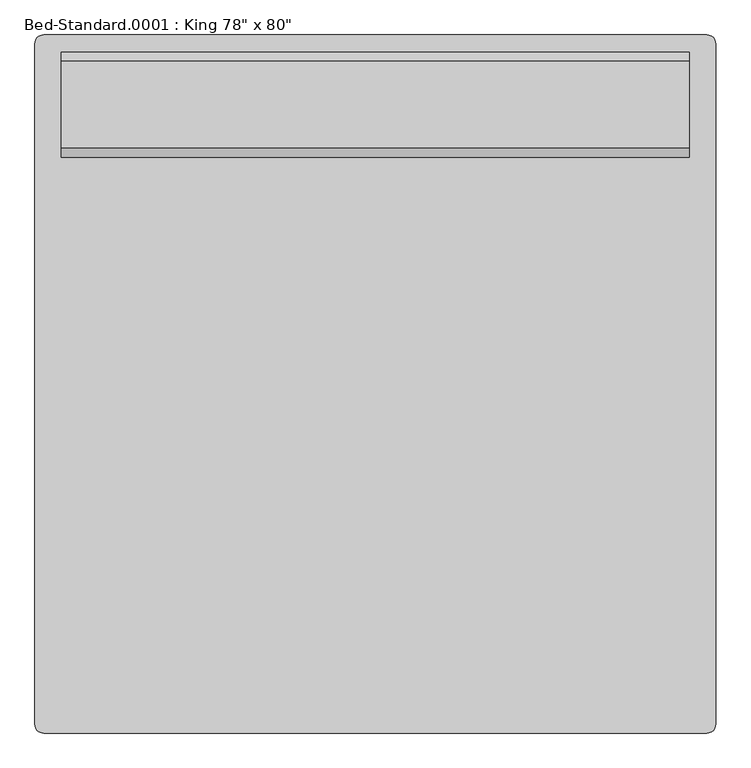
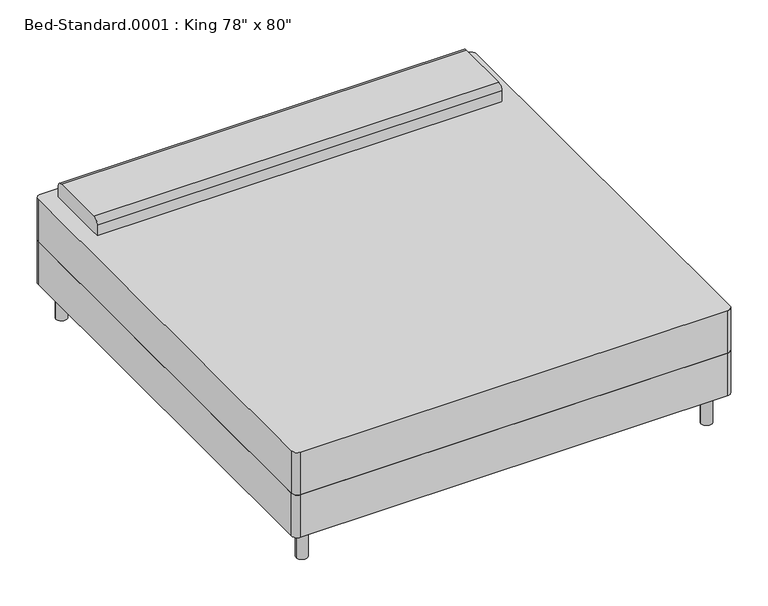
"""IFC4 building model written with IfcOpenShell, lengths in millimetres: furniture geometry."""

from ifc_helpers import new_model, si_unit, point, frame, frame_2d, origin, origin_with_axes, place, context, project, spatial, polyline, circle_curve, trimmed, segment, composite_curve, outline, extrude, source, transform, mapped, element, save


def furniture_1fc5af50(model_context):
    return source(origin(), model_context, "Body", "SweptSolid", [
        extrude(outline(composite_curve([segment(polyline([(-719.1114754, -1036.195082), (-719.1114754, 945.004918)]), True, "CONTINUOUS"), segment(trimmed(circle_curve(frame_2d((-693.7114754, 945.004918)), 25.4), [point((-719.1114754, 945.004918))], [point((-693.7114754, 970.404918))], False, "CARTESIAN"), True, "CONTINUOUS"), segment(polyline([(-693.7114754, 970.404918), (1236.6885246, 970.404918)]), True, "CONTINUOUS"), segment(trimmed(circle_curve(frame_2d((1236.6885246, 945.004918)), 25.4), [point((1236.6885246, 970.404918))], [point((1262.0885246, 945.004918))], False, "CARTESIAN"), True, "CONTINUOUS"), segment(polyline([(1262.0885246, 945.004918), (1262.0885246, -1036.195082)]), True, "CONTINUOUS"), segment(trimmed(circle_curve(frame_2d((1236.6885246, -1036.195082)), 25.4), [point((1262.0885246, -1036.195082))], [point((1236.6885246, -1061.595082))], False, "CARTESIAN"), True, "CONTINUOUS"), segment(polyline([(1236.6885246, -1061.595082), (-693.7114754, -1061.595082)]), True, "CONTINUOUS"), segment(trimmed(circle_curve(frame_2d((-693.7114754, -1036.195082)), 25.4), [point((-693.7114754, -1061.595082))], [point((-719.1114754, -1036.195082))], False, "CARTESIAN"), True, "CONTINUOUS")], self_intersect=False)), frame((0.0, 0.0, 152.4), z_axis=(0.0, 0.0, 1.0), x_axis=(1.0, 0.0, 0.0)), (0.0, 0.0, 1.0), 203.2),
        extrude(outline(composite_curve([segment(polyline([(614.804918, 558.8), (614.804918, 609.6)]), True, "CONTINUOUS"), segment(trimmed(circle_curve(frame_2d((640.204918, 609.6)), 25.4), [point((614.804918, 609.6))], [point((640.204918, 635.0))], False, "CARTESIAN"), True, "CONTINUOUS"), segment(polyline([(640.204918, 635.0), (894.204918, 635.0)]), True, "CONTINUOUS"), segment(trimmed(circle_curve(frame_2d((894.204918, 609.6)), 25.4), [point((894.204918, 635.0))], [point((919.604918, 609.6))], False, "CARTESIAN"), True, "CONTINUOUS"), segment(polyline([(919.604918, 609.6), (919.604918, 558.8), (614.804918, 558.8)]), True, "CONTINUOUS")], self_intersect=False)), frame((-642.9114754, 0.0, 0.0), z_axis=(1.0, 0.0, 0.0), x_axis=(0.0, 1.0, 0.0)), (0.0, 0.0, 1.0), 1828.8),
        extrude(outline(composite_curve([segment(trimmed(circle_curve(frame_2d((-642.9114754, 894.204918)), 25.4), [point((-668.3114754, 894.204918))], [point((-617.5114754, 894.204918))], False, "CARTESIAN"), True, "CONTINUOUS"), segment(trimmed(circle_curve(frame_2d((-642.9114754, 894.204918)), 25.4), [point((-617.5114754, 894.204918))], [point((-668.3114754, 894.204918))], False, "CARTESIAN"), True, "CONTINUOUS")], self_intersect=False)), origin_with_axes(), (0.0, 0.0, 1.0), 152.4),
        extrude(outline(composite_curve([segment(trimmed(circle_curve(frame_2d((1185.8885246, 894.204918)), 25.4), [point((1160.4885246, 894.204918))], [point((1211.2885246, 894.204918))], False, "CARTESIAN"), True, "CONTINUOUS"), segment(trimmed(circle_curve(frame_2d((1185.8885246, 894.204918)), 25.4), [point((1211.2885246, 894.204918))], [point((1160.4885246, 894.204918))], False, "CARTESIAN"), True, "CONTINUOUS")], self_intersect=False)), origin_with_axes(), (0.0, 0.0, 1.0), 152.4),
        extrude(outline(composite_curve([segment(trimmed(circle_curve(frame_2d((1185.8885246, -985.395082)), 25.4), [point((1160.4885246, -985.395082))], [point((1211.2885246, -985.395082))], False, "CARTESIAN"), True, "CONTINUOUS"), segment(trimmed(circle_curve(frame_2d((1185.8885246, -985.395082)), 25.4), [point((1211.2885246, -985.395082))], [point((1160.4885246, -985.395082))], False, "CARTESIAN"), True, "CONTINUOUS")], self_intersect=False)), origin_with_axes(), (0.0, 0.0, 1.0), 152.4),
        extrude(outline(composite_curve([segment(trimmed(circle_curve(frame_2d((-642.9114754, -985.395082)), 25.4), [point((-668.3114754, -985.395082))], [point((-617.5114754, -985.395082))], False, "CARTESIAN"), True, "CONTINUOUS"), segment(trimmed(circle_curve(frame_2d((-642.9114754, -985.395082)), 25.4), [point((-617.5114754, -985.395082))], [point((-668.3114754, -985.395082))], False, "CARTESIAN"), True, "CONTINUOUS")], self_intersect=False)), origin_with_axes(), (0.0, 0.0, 1.0), 152.4),
        extrude(outline(composite_curve([segment(polyline([(-693.7114754, 970.404918), (1236.6885246, 970.404918)]), True, "CONTINUOUS"), segment(trimmed(circle_curve(frame_2d((1236.6885246, 945.004918)), 25.4), [point((1236.6885246, 970.404918))], [point((1262.0885246, 945.004918))], False, "CARTESIAN"), True, "CONTINUOUS"), segment(polyline([(1262.0885246, 945.004918), (1262.0885246, -1036.195082)]), True, "CONTINUOUS"), segment(trimmed(circle_curve(frame_2d((1236.6885246, -1036.195082)), 25.4), [point((1262.0885246, -1036.195082))], [point((1236.6885246, -1061.595082))], False, "CARTESIAN"), True, "CONTINUOUS"), segment(polyline([(1236.6885246, -1061.595082), (-693.7114754, -1061.595082)]), True, "CONTINUOUS"), segment(trimmed(circle_curve(frame_2d((-693.7114754, -1036.195082)), 25.4), [point((-693.7114754, -1061.595082))], [point((-719.1114754, -1036.195082))], False, "CARTESIAN"), True, "CONTINUOUS"), segment(polyline([(-719.1114754, -1036.195082), (-719.1114754, 945.004918)]), True, "CONTINUOUS"), segment(trimmed(circle_curve(frame_2d((-693.7114754, 945.004918)), 25.4), [point((-719.1114754, 945.004918))], [point((-693.7114754, 970.404918))], False, "CARTESIAN"), True, "CONTINUOUS")], self_intersect=False)), frame((0.0, 0.0, 355.6), z_axis=(0.0, 0.0, 1.0), x_axis=(1.0, 0.0, 0.0)), (0.0, 0.0, 1.0), 203.2),
    ])


if __name__ == "__main__":
    model = new_model("IFC4")
    model_context = context("Model", 3, world=origin())
    ifc_project = project(units=[si_unit("LENGTHUNIT", "METRE", prefix="MILLI")], contexts=[model_context])
    site = spatial("IfcSite", under=ifc_project)
    building = spatial("IfcBuilding", under=site)
    placement = place(None, origin())
    furniture_shape = furniture_1fc5af50(model_context)
    element("IfcFurniture", 1, ObjectType="Bed-Standard.0001 : King 78\" x 80\"", at=placement, inside=building, context=model_context, shape_type="MappedRepresentation", body=[
        mapped(furniture_shape, transform((0.0, 0.0, 0.0), x_axis=(1.0, 0.0, 0.0), y_axis=(0.0, 1.0, 0.0), z_axis=(0.0, 0.0, 1.0))),
    ])
    save(model, "model.ifc")

# Revit data of these elements
# Type "Bed-Standard.0001 : King 78\" x 80\""
#   Assembly Code = "E2020200"
#   Length = 6' - 8"
#   Width = 6' - 6"
#   Leg Material = Steel, Chrome Plated
#   Mattress Material = Softwood, Lumber
#   Default Elevation = 0
# Element 1 (IfcFurniture, "Bed-Standard.0001 : King 78\" x 80\"")
#   Materials on its faces: "Linen, White", "Steel, Chrome Plated"
# Materials
#   "Steel, Chrome Plated": class "Metal", colour RGB 17 17 17, transparency 0, Description = "Chromiuim plated steel", Cost = 0
#   "Softwood, Lumber": class "Wood", colour RGB 223 192 134, transparency 0, Description = "Pinus Echinata", Cost = 0
#   "Linen, White": class "Textile", colour RGB 247 247 239, transparency 0, Description = "Linen, white", Cost = 0
